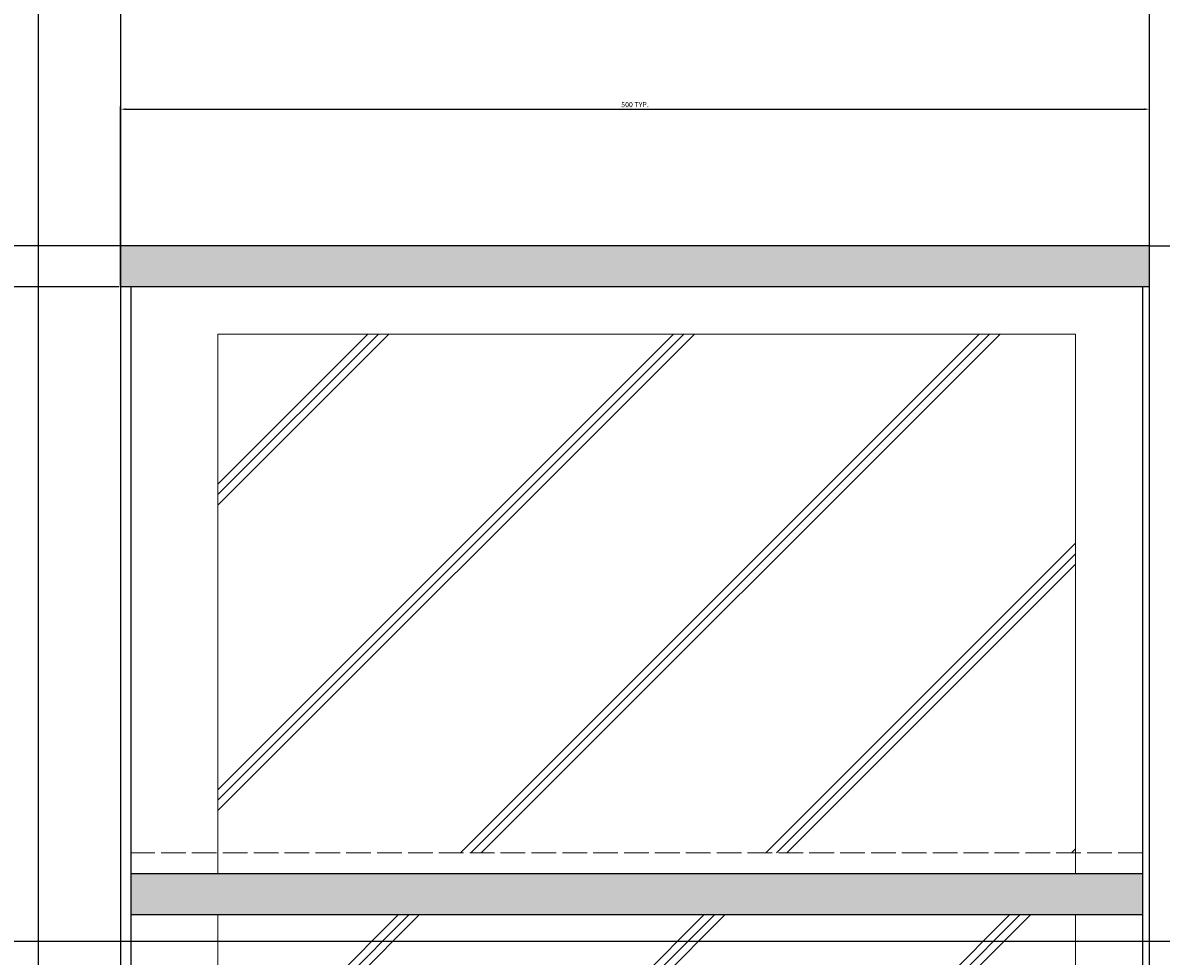
# Model space of a CAD drawing. Units: millimetres. Extents: x 2332 to 5836, y -853 to 2199.
# Tile 4 of 16: x 3088 to 3641, y 1023 to 1476. Entities that reach past the tile are written whole.
import ezdxf

# ---------------------------------------------------------------- set-up
doc = ezdxf.new("R2010")
doc.units = ezdxf.units.MM
doc.linetypes.add('ACAD_ISO02W100', pattern=[15, 12, -3])
doc.layers.get('0').update_dxf_attribs({"color": 8})
for name, color, linetype, lineweight in [('A-ANNO-DIMS', 2, 'Continuous', 18), ('A-CSWK-GLAZ', 7, 'Continuous', 18), ('A-CSWK-HIDN', 8, 'ACAD_ISO02W100', 13), ('A-CSWK-PATT', 40, 'Continuous', 13), ('A-GLAZ-PATT', 4, 'Continuous', 13), ('SHELF', 40, 'Continuous', 25)]:
    doc.layers.add(name, color=color, linetype=linetype, lineweight=lineweight)
doc.styles.get("Standard").update_dxf_attribs({"font": 'arial.ttf'})
doc.dimstyles.new('ISO-25', dxfattribs={"dimtxt": 2.5, "dimasz": 2.5, "dimexe": 1.25, "dimexo": 0.625, "dimtad": 1, "dimtxsty": 'Standard', "dimcen": 2.5, "dimadec": 0, "dimazin": 0, "dimtfac": 1, "dimtmove": 0, "dimatfit": 3, "dimfxl": 1, "dimarcsym": 0})

# ---------------------------------------------------------------- blocks, each defined once
blk = doc.blocks.new('CAB-END-STILE')
blk.add_line((113.09, 1240), (113.09, 0))
blk = doc.blocks.new('CAB-GLAZED-FACE-FRAME')
for p, q in [((500, 575.53), (0, 575.53)), ((5, 575.53), (5, 0)), ((496.71, 0), (496.71, 575.53)), ((5, 0), (496.71, 0))]:
    blk.add_line(p, q)
blk = doc.blocks.new('*D13')
at = {"layer": 'A-ANNO-DIMS', "color": 0, "lineweight": -2, "transparency": 16777216}
for p, q in [((3134.41, 1347.8), (3047.46, 1347.8)), ((3048.71, 774.77), (3048.71, 1345.3)), ((3134.41, 772.27), (3047.46, 772.27))]:
    blk.add_line(p, q, dxfattribs=at)
at = {"layer": 'A-ANNO-DIMS', "color": 0, "transparency": 16777216}
for points in [[(3048.29, 1345.3), (3049.13, 1345.3), (3048.71, 1347.8)], [(3048.29, 774.77), (3049.13, 774.77), (3048.71, 772.27)]]:
    blk.add_solid(points, dxfattribs=at)
at = {"layer": 'Defpoints', "color": 0, "transparency": 16777216}
for p in [(3048.71, 1347.8), (3135.04, 1347.8), (3135.04, 772.27)]:
    blk.add_point(p, dxfattribs=at)
at = {"layer": 'A-ANNO-DIMS', "color": 0, "transparency": 16777216, "insert": (3046.79, 1060.04), "char_height": 2.5, "attachment_point": 5, "rotation": 90}
blk.add_mtext('GLAZED FRAME 576 TYP.', dxfattribs=at)
blk = doc.blocks.new('*D14')
at = {"layer": 'A-ANNO-DIMS', "color": 0, "lineweight": -2, "transparency": 16777216}
for p, q in [((3135.04, 1348.43), (3135.04, 1435.38)), ((3137.54, 1434.13), (3632.54, 1434.13)), ((3635.04, 1348.43), (3635.04, 1435.38))]:
    blk.add_line(p, q, dxfattribs=at)
at = {"layer": 'A-ANNO-DIMS', "color": 0, "transparency": 16777216}
for points in [[(3137.54, 1434.55), (3137.54, 1433.72), (3135.04, 1434.13)], [(3632.54, 1434.55), (3632.54, 1433.72), (3635.04, 1434.13)]]:
    blk.add_solid(points, dxfattribs=at)
at = {"layer": 'Defpoints', "color": 0, "transparency": 16777216}
for p in [(3635.04, 1434.13), (3135.04, 1347.8), (3635.04, 1347.8)]:
    blk.add_point(p, dxfattribs=at)
at = {"layer": 'A-ANNO-DIMS', "color": 0, "transparency": 16777216, "insert": (3385.04, 1436.04), "char_height": 2.5, "attachment_point": 5}
blk.add_mtext('500 TYP.', dxfattribs=at)
blk = doc.blocks.new('*D29')
at = {"layer": 'A-ANNO-DIMS', "color": 0, "lineweight": -2, "transparency": 16777216}
for p, q in [((3634.41, 1367.8), (2334.14, 1367.8)), ((2335.39, 1032.3), (2335.39, 1365.3)), ((3645.84, 1029.8), (2334.14, 1029.8))]:
    blk.add_line(p, q, dxfattribs=at)
at = {"layer": 'A-ANNO-DIMS', "color": 0, "transparency": 16777216}
for points in [[(2334.97, 1365.3), (2335.81, 1365.3), (2335.39, 1367.8)], [(2334.97, 1032.3), (2335.81, 1032.3), (2335.39, 1029.8)]]:
    blk.add_solid(points, dxfattribs=at)
at = {"layer": 'Defpoints', "color": 0, "transparency": 16777216}
for p in [(2335.39, 1367.8), (3635.04, 1367.8), (3646.47, 1029.8)]:
    blk.add_point(p, dxfattribs=at)
at = {"layer": 'A-ANNO-DIMS', "color": 0, "transparency": 16777216, "insert": (2333.49, 1198.8), "char_height": 2.5, "attachment_point": 5, "rotation": 90}
blk.add_mtext('338', dxfattribs=at)
blk = doc.blocks.new('*D30')
at = {"layer": 'A-ANNO-DIMS', "color": 0, "lineweight": -2, "transparency": 16777216}
for p, q in [((3635.04, 1368.43), (3635.04, 2168.7)), ((4210.04, 1368.43), (4210.04, 2168.7)), ((3637.54, 2167.45), (4207.54, 2167.45))]:
    blk.add_line(p, q, dxfattribs=at)
at = {"layer": 'A-ANNO-DIMS', "color": 0, "transparency": 16777216}
for points in [[(3637.54, 2167.87), (3637.54, 2167.04), (3635.04, 2167.45)], [(4207.54, 2167.87), (4207.54, 2167.04), (4210.04, 2167.45)]]:
    blk.add_solid(points, dxfattribs=at)
at = {"layer": 'Defpoints', "color": 0, "transparency": 16777216}
for p in [(4210.04, 2167.45), (3635.04, 1367.8), (4210.04, 1367.8)]:
    blk.add_point(p, dxfattribs=at)
at = {"layer": 'A-ANNO-DIMS', "color": 0, "transparency": 16777216, "insert": (3922.54, 2169.35), "char_height": 2.5, "attachment_point": 5}
blk.add_mtext('575', dxfattribs=at)

msp = doc.modelspace()

# ---------------------------------------------------------------- hatches: boundary and pattern name
at = {"layer": 'A-CSWK-PATT'}
h = msp.add_hatch(color=256, dxfattribs=at)
h.dxf.hatch_style = 1
h.paths.add_polyline_path([(3635.04, 1367.803), (3135.04, 1367.803), (3135.04, 1347.803), (3635.04, 1347.803)])
h.paths.add_polyline_path([(3599.069, 1062.803), (3182.349, 1062.803), (3182.349, 1042.803), (3599.069, 1042.803)])
h.paths.add_polyline_path([(3182.349, 1062.803), (3140.04, 1062.803), (3140.04, 1042.803), (3182.349, 1042.803)])
h.paths.add_polyline_path([(3631.75, 1062.803), (3599.069, 1062.803), (3599.069, 1042.803), (3631.75, 1042.803)])
at = {"layer": 'A-GLAZ-PATT'}
h = msp.add_hatch(dxfattribs=at)
h.set_pattern_fill('JIS_RC_15', color=256, scale=7)
h.paths.add_polyline_path([(3599.069, 1324.883), (3182.349, 1324.883), (3182.349, 1072.803), (3599.069, 1072.803)])
h.paths.add_polyline_path([(3599.069, 1042.803), (3182.349, 1042.803), (3182.349, 813.86), (3599.069, 813.86)])

# ---------------------------------------------------------------- linework, layer by layer
at = {"layer": 'A-CSWK-GLAZ'}
for points in [[(3182.349, 1062.803), (3182.349, 1324.883), (3599.069, 1324.883), (3599.069, 1062.803)], [(3599.069, 1042.803), (3599.069, 813.86), (3182.349, 813.86), (3182.349, 1042.803)]]:
    msp.add_lwpolyline(points, dxfattribs=at)
at = {"layer": 'A-CSWK-HIDN'}
msp.add_line((3631.75, 1072.803), (3140.04, 1072.803), dxfattribs=at)
at = {"layer": 'SHELF'}
for p, q in [((3135.04, 1967.803), (3135.04, 767.803)), ((3635.04, 767.803), (3635.04, 1967.803)), ((3635.04, 1367.803), (2745.04, 1367.803)), ((3635.04, 1367.803), (4785.04, 1367.803)), ((3140.04, 1062.803), (3631.75, 1062.803)), ((3140.04, 1042.803), (3631.75, 1042.803))]:
    msp.add_line(p, q, dxfattribs=at)

# ---------------------------------------------------------------- block references
for name, p in [('CAB-END-STILE', (2981.95, 767.803)), ('CAB-GLAZED-FACE-FRAME', (3135.04, 772.269))]:
    msp.add_blockref(name, p, dxfattribs=at)

# ---------------------------------------------------------------- dimensions: what is measured, and where the dimension line sits
at = {"layer": 'A-ANNO-DIMS'}
dim = msp.add_linear_dim(base=(4210.04, 2167.453), p1=(3635.04, 1367.803), p2=(4210.04, 1367.803), dimstyle='ISO-25', override={"dimdec": 0, "dimlfac": 1, "dimrnd": 0, "dimzin": 0, "dimdsep": 46, "dimlunit": 2}, dxfattribs=at)
dim.commit()
dim.dimension.update_dxf_attribs({"geometry": '*D30', "text_midpoint": (3922.54, 2169.35)})
dim = msp.add_linear_dim(base=(3635.04, 1434.134), p1=(3135.04, 1347.803), p2=(3635.04, 1347.803), text='<> TYP.', dimstyle='ISO-25', override={"dimdec": 0, "dimlfac": 1, "dimrnd": 0, "dimzin": 0, "dimdsep": 46, "dimlunit": 2}, dxfattribs=at)
dim.commit()
dim.dimension.update_dxf_attribs({"geometry": '*D14', "text_midpoint": (3385.04, 1436.035)})
dim = msp.add_linear_dim(base=(2335.39, 1367.803), p1=(3646.468, 1029.801), p2=(3635.04, 1367.803), angle=90, dimstyle='ISO-25', override={"dimdec": 0, "dimlfac": 1, "dimrnd": 0, "dimzin": 0, "dimdsep": 46, "dimlunit": 2}, dxfattribs=at)
dim.commit()
dim.dimension.update_dxf_attribs({"geometry": '*D29', "text_midpoint": (2333.488, 1198.802)})
dim = msp.add_linear_dim(base=(3048.71, 1347.803), p1=(3135.04, 772.269), p2=(3135.04, 1347.803), angle=90, text='GLAZED FRAME <> TYP.', dimstyle='ISO-25', override={"dimdec": 0, "dimlfac": 1, "dimrnd": 0, "dimzin": 0, "dimdsep": 46, "dimlunit": 2}, dxfattribs=at)
dim.commit()
dim.dimension.update_dxf_attribs({"geometry": '*D13', "text_midpoint": (3046.792, 1060.036)})

doc.saveas('drawing.dxf')
